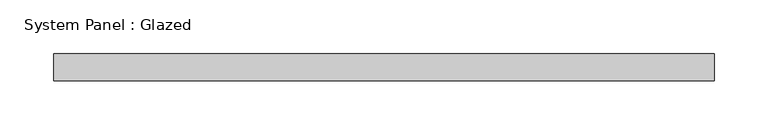
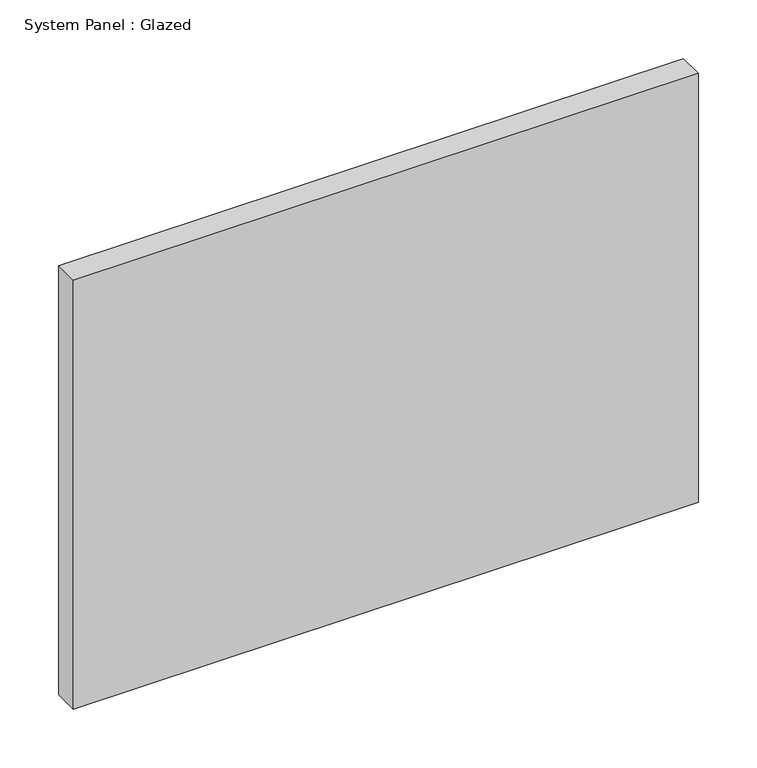
"""IFC4 building model written with IfcOpenShell, lengths in millimetres: plate geometry, System Panel : Glazed."""

from ifc_helpers import new_model, si_unit, origin, origin_with_axes, place, context, project, spatial, polyline, outline, extrude, source, transform, mapped, element, save


def system_panel_glazed_e2a89770(model_context):
    return source(origin(), model_context, "Body", "SweptSolid", [
        extrude(outline(polyline([(307.975, 19.05), (-307.975, 19.05), (-307.975, 44.45), (307.975, 44.45), (307.975, 19.05)])), origin_with_axes(), (0.0, 0.0, 1.0), 446.9248327),
    ])


if __name__ == "__main__":
    model = new_model("IFC4")
    model_context = context("Model", 3, world=origin())
    ifc_project = project(units=[si_unit("LENGTHUNIT", "METRE", prefix="MILLI")], contexts=[model_context])
    site = spatial("IfcSite", under=ifc_project)
    building = spatial("IfcBuilding", under=site)
    placement = place(None, origin())
    system_panel_glazed_shape = system_panel_glazed_e2a89770(model_context)
    element("IfcPlate", 1, ObjectType="System Panel : Glazed", at=placement, inside=building, context=model_context, shape_type="MappedRepresentation", body=[
        mapped(system_panel_glazed_shape, transform((0.0, 0.0, 0.0), x_axis=(1.0, 0.0, 0.0), y_axis=(0.0, 1.0, 0.0), z_axis=(0.0, 0.0, 1.0))),
    ])
    save(model, "model.ifc")

# Revit data of these elements
# Type "System Panel : Glazed"
#   Construction Type Id = "GSP4R"
#   Analytic Construction = "1/8 in Pilkington single glazing"
#   Visual Light Transmittance = 0.9
#   Solar Heat Gain Coefficient = 0.86
#   Heat Transfer Coefficient (U) = 1.18115 BTU/(h·ft²·°F)
#   Define Thermal Properties by = 1
# Element 1 (IfcPlate, "System Panel : Glazed")
#   Materials on its faces: "Glass"
# Materials
#   "Glass": class "Glass", colour RGB 0 128 192, transparency 0.75, Description = "Soda Lime Glass", Cost = 0
